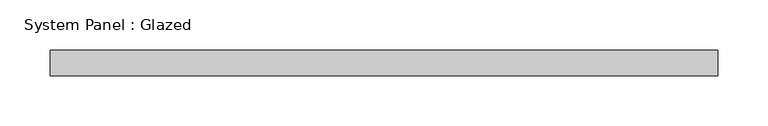
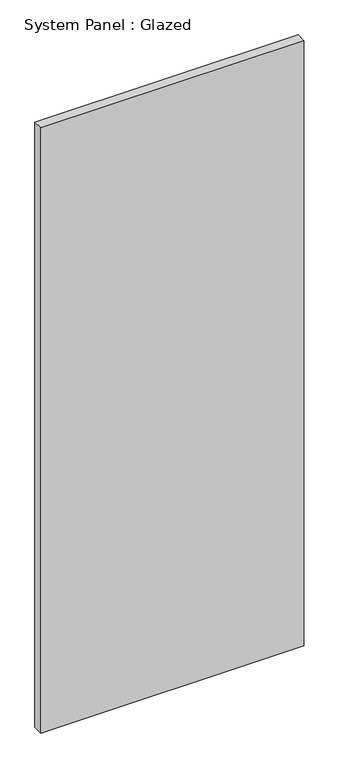
"""IFC4 building model written with IfcOpenShell, lengths in millimetres: plate geometry, System Panel : Glazed."""

from ifc_helpers import new_model, si_unit, origin, origin_with_axes, place, context, project, spatial, polyline, outline, extrude, source, transform, mapped, element, save


def system_panel_glazed_dddf758e(model_context):
    return source(origin(), model_context, "Body", "SweptSolid", [
        extrude(outline(polyline([(333.375, 19.05), (-333.375, 19.05), (-333.375, 44.45), (333.375, 44.45), (333.375, 19.05)])), origin_with_axes(), (0.0, 0.0, 1.0), 1621.0218004),
    ])


if __name__ == "__main__":
    model = new_model("IFC4")
    model_context = context("Model", 3, world=origin())
    ifc_project = project(units=[si_unit("LENGTHUNIT", "METRE", prefix="MILLI")], contexts=[model_context])
    site = spatial("IfcSite", under=ifc_project)
    building = spatial("IfcBuilding", under=site)
    placement = place(None, origin())
    system_panel_glazed_shape = system_panel_glazed_dddf758e(model_context)
    element("IfcPlate", 1, ObjectType="System Panel : Glazed", at=placement, inside=building, context=model_context, shape_type="MappedRepresentation", body=[
        mapped(system_panel_glazed_shape, transform((0.0, 0.0, 0.0), x_axis=(1.0, 0.0, 0.0), y_axis=(0.0, 1.0, 0.0), z_axis=(0.0, 0.0, 1.0))),
    ])
    save(model, "model.ifc")

# Revit data of these elements
# Type "System Panel : Glazed"
#   Construction Type Id = "GSP4R"
#   Analytic Construction = "1/8 in Pilkington single glazing"
#   Visual Light Transmittance = 0.9
#   Solar Heat Gain Coefficient = 0.86
#   Heat Transfer Coefficient (U) = 1.18115 BTU/(h·ft²·°F)
#   Define Thermal Properties by = 1
# Element 1 (IfcPlate, "System Panel : Glazed")
#   Materials on its faces: "Glass"
# Materials
#   "Glass": class "Glass", colour RGB 0 128 192, transparency 0.75, Description = "Soda Lime Glass", Cost = 0
